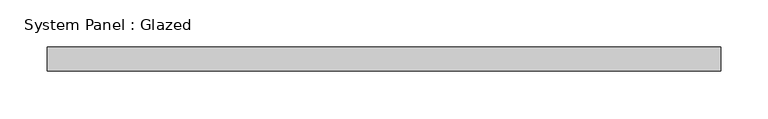
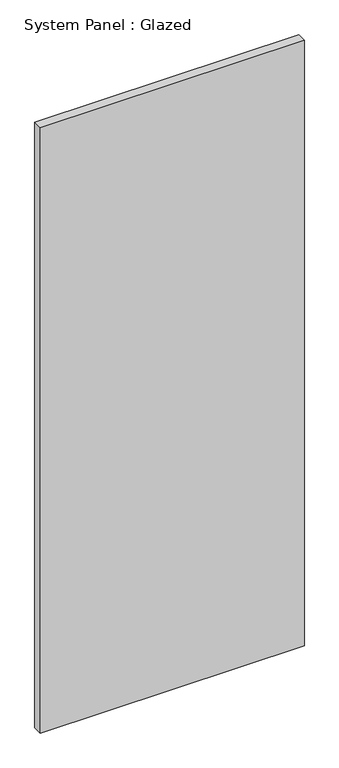
"""IFC4 building model written with IfcOpenShell, lengths in millimetres: plate geometry, System Panel : Glazed."""

from ifc_helpers import new_model, si_unit, origin, origin_with_axes, place, context, project, spatial, polyline, outline, extrude, source, transform, mapped, element, save


def system_panel_glazed_23071c8f(model_context):
    return source(origin(), model_context, "Body", "SweptSolid", [
        extrude(outline(polyline([(355.6, 19.05), (-355.6, 19.05), (-355.6, 44.45), (355.6, 44.45), (355.6, 19.05)])), origin_with_axes(), (0.0, 0.0, 1.0), 1722.9041833),
    ])


if __name__ == "__main__":
    model = new_model("IFC4")
    model_context = context("Model", 3, world=origin())
    ifc_project = project(units=[si_unit("LENGTHUNIT", "METRE", prefix="MILLI")], contexts=[model_context])
    site = spatial("IfcSite", under=ifc_project)
    building = spatial("IfcBuilding", under=site)
    placement = place(None, origin())
    system_panel_glazed_shape = system_panel_glazed_23071c8f(model_context)
    element("IfcPlate", 1, ObjectType="System Panel : Glazed", at=placement, inside=building, context=model_context, shape_type="MappedRepresentation", body=[
        mapped(system_panel_glazed_shape, transform((0.0, 0.0, 0.0), x_axis=(1.0, 0.0, 0.0), y_axis=(0.0, 1.0, 0.0), z_axis=(0.0, 0.0, 1.0))),
    ])
    save(model, "model.ifc")

# Revit data of these elements
# Type "System Panel : Glazed"
#   Construction Type Id = "GSP4R"
#   Analytic Construction = "1/8 in Pilkington single glazing"
#   Visual Light Transmittance = 0.9
#   Solar Heat Gain Coefficient = 0.86
#   Heat Transfer Coefficient (U) = 1.18115 BTU/(h·ft²·°F)
# Element 1 (IfcPlate, "System Panel : Glazed")
#   Materials on its faces: "Glass"
# Materials
#   "Glass": class "Glass", colour RGB 0 128 192, transparency 0.75, Description = "Soda Lime Glass", Cost = 0
